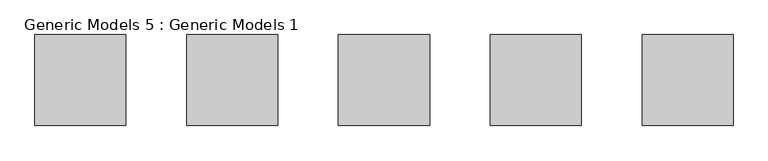
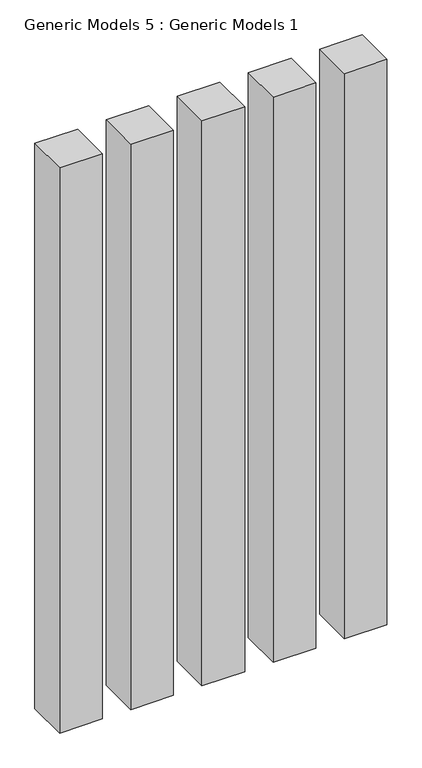
"""IFC4 building model written with IfcOpenShell, lengths in millimetres: proxy geometry, Generic Models 5 : Generic Models 1."""

from ifc_helpers import new_model, si_unit, origin, origin_with_axes, place, context, project, spatial, polyline, outline, extrude, source, transform, mapped, element, save


def generic_models_5_generic_models_1_cca4fb08(model_context):
    return source(origin(), model_context, "Body", "SweptSolid", [
        extrude(outline(polyline([(-13871.5453682, 12607.034892), (-13871.5453682, 12378.434892), (-14100.1453682, 12378.434892), (-14100.1453682, 12607.034892), (-13871.5453682, 12607.034892)])), origin_with_axes(), (0.0, 0.0, 1.0), 3200.4),
        extrude(outline(polyline([(-13490.5453682, 12607.034892), (-13490.5453682, 12378.434892), (-13719.1453682, 12378.434892), (-13719.1453682, 12607.034892), (-13490.5453682, 12607.034892)])), origin_with_axes(), (0.0, 0.0, 1.0), 3200.4),
        extrude(outline(polyline([(-13109.5453682, 12607.034892), (-13109.5453682, 12378.434892), (-13338.1453682, 12378.434892), (-13338.1453682, 12607.034892), (-13109.5453682, 12607.034892)])), origin_with_axes(), (0.0, 0.0, 1.0), 3200.4),
        extrude(outline(polyline([(-12728.5453682, 12607.034892), (-12728.5453682, 12378.434892), (-12957.1453682, 12378.434892), (-12957.1453682, 12607.034892), (-12728.5453682, 12607.034892)])), origin_with_axes(), (0.0, 0.0, 1.0), 3200.4),
        extrude(outline(polyline([(-12347.5453682, 12607.034892), (-12347.5453682, 12378.434892), (-12576.1453682, 12378.434892), (-12576.1453682, 12607.034892), (-12347.5453682, 12607.034892)])), origin_with_axes(), (0.0, 0.0, 1.0), 3200.4),
    ])


if __name__ == "__main__":
    model = new_model("IFC4")
    model_context = context("Model", 3, world=origin())
    ifc_project = project(units=[si_unit("LENGTHUNIT", "METRE", prefix="MILLI")], contexts=[model_context])
    site = spatial("IfcSite", under=ifc_project)
    building = spatial("IfcBuilding", under=site)
    placement = place(None, origin())
    generic_models_5_generic_models_1_shape = generic_models_5_generic_models_1_cca4fb08(model_context)
    element("IfcBuildingElementProxy", 1, Name="Generic Models 5 : Generic Models 1", ObjectType="Generic Models 5 : Generic Models 1", at=placement, inside=building, context=model_context, shape_type="MappedRepresentation", body=[
        mapped(generic_models_5_generic_models_1_shape, transform((0.0, 0.0, 0.0), x_axis=(1.0, 0.0, 0.0), y_axis=(0.0, 1.0, 0.0), z_axis=(0.0, 0.0, 1.0))),
    ])
    save(model, "model.ifc")

# Revit data of these elements
# Element 1 (IfcBuildingElementProxy, "Generic Models 5 : Generic Models 1")
#   Materials on its faces: "0 olive green"
# Materials
#   "0 olive green": class "Generic", colour RGB 120 120 120, transparency 0, Cost = 0
